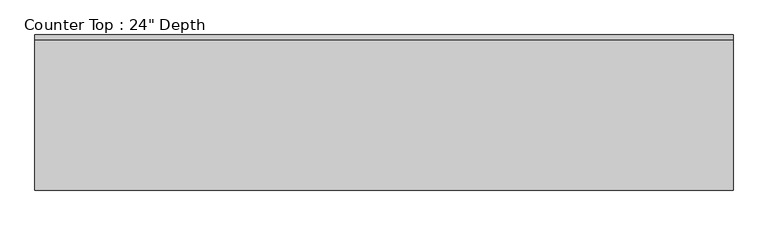
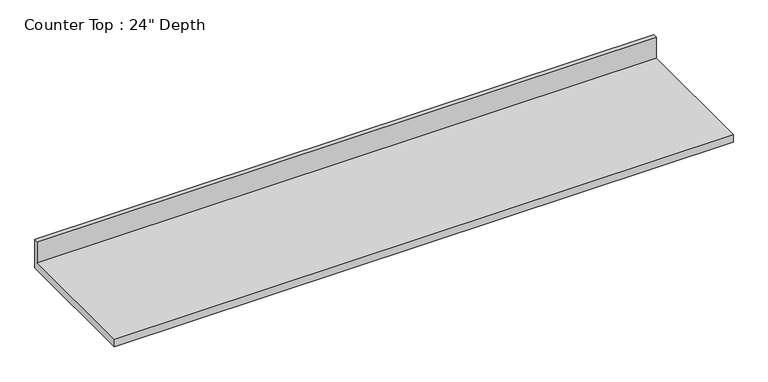
"""IFC4 building model written with IfcOpenShell, lengths in millimetres: furniture geometry."""

from ifc_helpers import new_model, si_unit, frame, origin, place, context, project, spatial, polyline, outline, extrude, source, transform, mapped, element, save


def furniture_7591947b(model_context):
    return source(origin(), model_context, "Body", "SweptSolid", [
        extrude(outline(polyline([(0.0, 1016.0), (0.0, 876.3), (-635.0, 876.3), (-635.0, 914.4), (-19.05, 914.4), (-19.05, 1016.0), (0.0, 1016.0)])), frame((-1200.4622951, 0.0, 0.0), z_axis=(1.0, 0.0, 0.0), x_axis=(0.0, 1.0, 0.0)), (0.0, 0.0, 1.0), 2857.5),
    ])


if __name__ == "__main__":
    model = new_model("IFC4")
    model_context = context("Model", 3, world=origin())
    ifc_project = project(units=[si_unit("LENGTHUNIT", "METRE", prefix="MILLI")], contexts=[model_context])
    site = spatial("IfcSite", under=ifc_project)
    building = spatial("IfcBuilding", under=site)
    placement = place(None, origin())
    furniture_shape = furniture_7591947b(model_context)
    element("IfcFurniture", 1, ObjectType="Counter Top : 24\" Depth", at=placement, inside=building, context=model_context, shape_type="MappedRepresentation", body=[
        mapped(furniture_shape, transform((0.0, 0.0, 0.0), x_axis=(1.0, 0.0, 0.0), y_axis=(0.0, 1.0, 0.0), z_axis=(0.0, 0.0, 1.0))),
    ])
    save(model, "model.ifc")

# Revit data of these elements
# Type "Counter Top : 24\" Depth"
#   Assembly Code = "C1030400"
#   Counter Thickness = 0' - 1 1/2"
#   Depth = 2' - 1"
#   Height = 3' - 0"
#   Length [instance default] = 8' - 0"
#   Counter Top Material = none
#   Default Elevation = 0
# Element 1 (IfcFurniture, "Counter Top : 24\" Depth")
#   Length = 9' - 4 1/2"
#   Materials on its faces: "Counter Top"
# Materials
#   "Counter Top": class "Wood", colour RGB 226 177 128, transparency 0
